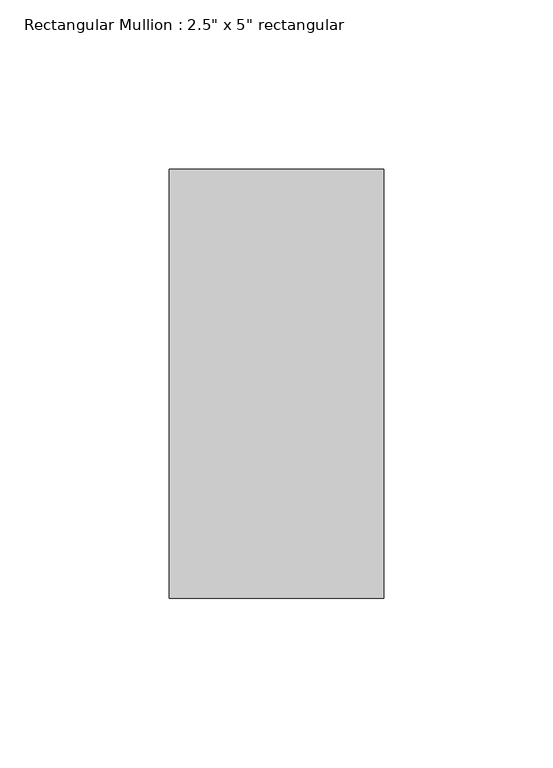
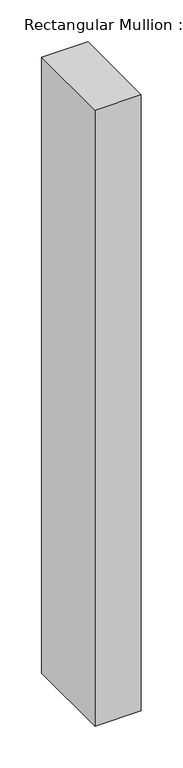
"""IFC4 building model written with IfcOpenShell, lengths in millimetres: member geometry."""

from ifc_helpers import new_model, si_unit, frame, origin, place, context, project, spatial, polyline, outline, extrude, source, transform, mapped, element, save


def member_f1f71bde(model_context):
    return source(origin(), model_context, "Body", "SweptSolid", [
        extrude(outline(polyline([(0.0, 63.5), (0.0, -63.5), (-63.5, -63.5), (-63.5, 63.5), (0.0, 63.5)])), frame((0.0, 0.0, -895.35), z_axis=(0.0, 0.0, 1.0), x_axis=(1.0, 0.0, 0.0)), (0.0, 0.0, 1.0), 895.35),
    ])


if __name__ == "__main__":
    model = new_model("IFC4")
    model_context = context("Model", 3, world=origin())
    ifc_project = project(units=[si_unit("LENGTHUNIT", "METRE", prefix="MILLI")], contexts=[model_context])
    site = spatial("IfcSite", under=ifc_project)
    building = spatial("IfcBuilding", under=site)
    placement = place(None, origin())
    member_shape = member_f1f71bde(model_context)
    element("IfcMember", 1, ObjectType="Rectangular Mullion : 2.5\" x 5\" rectangular", at=placement, inside=building, context=model_context, shape_type="MappedRepresentation", body=[
        mapped(member_shape, transform((0.0, 0.0, 0.0), x_axis=(1.0, 0.0, 0.0), y_axis=(0.0, 1.0, 0.0), z_axis=(0.0, 0.0, 1.0))),
    ])
    save(model, "model.ifc")

# Revit data of these elements
# Type "Rectangular Mullion : 2.5\" x 5\" rectangular"
#   built-in parameter 1007304 = 0.416667 (stored number, unit not read)
#   built-in parameter 1007301 = 0.104167 (stored number, unit not read)
#   built-in parameter 1007300 = 0.104167 (stored number, unit not read)
# Element 1 (IfcMember, "Rectangular Mullion : 2.5\" x 5\" rectangular")
#   Materials on its faces: "Aluminum"
# Materials
#   "Aluminum": class "Metal", colour RGB 247 247 247, transparency 0, Description = "Aluminum 6061", Cost = 0
